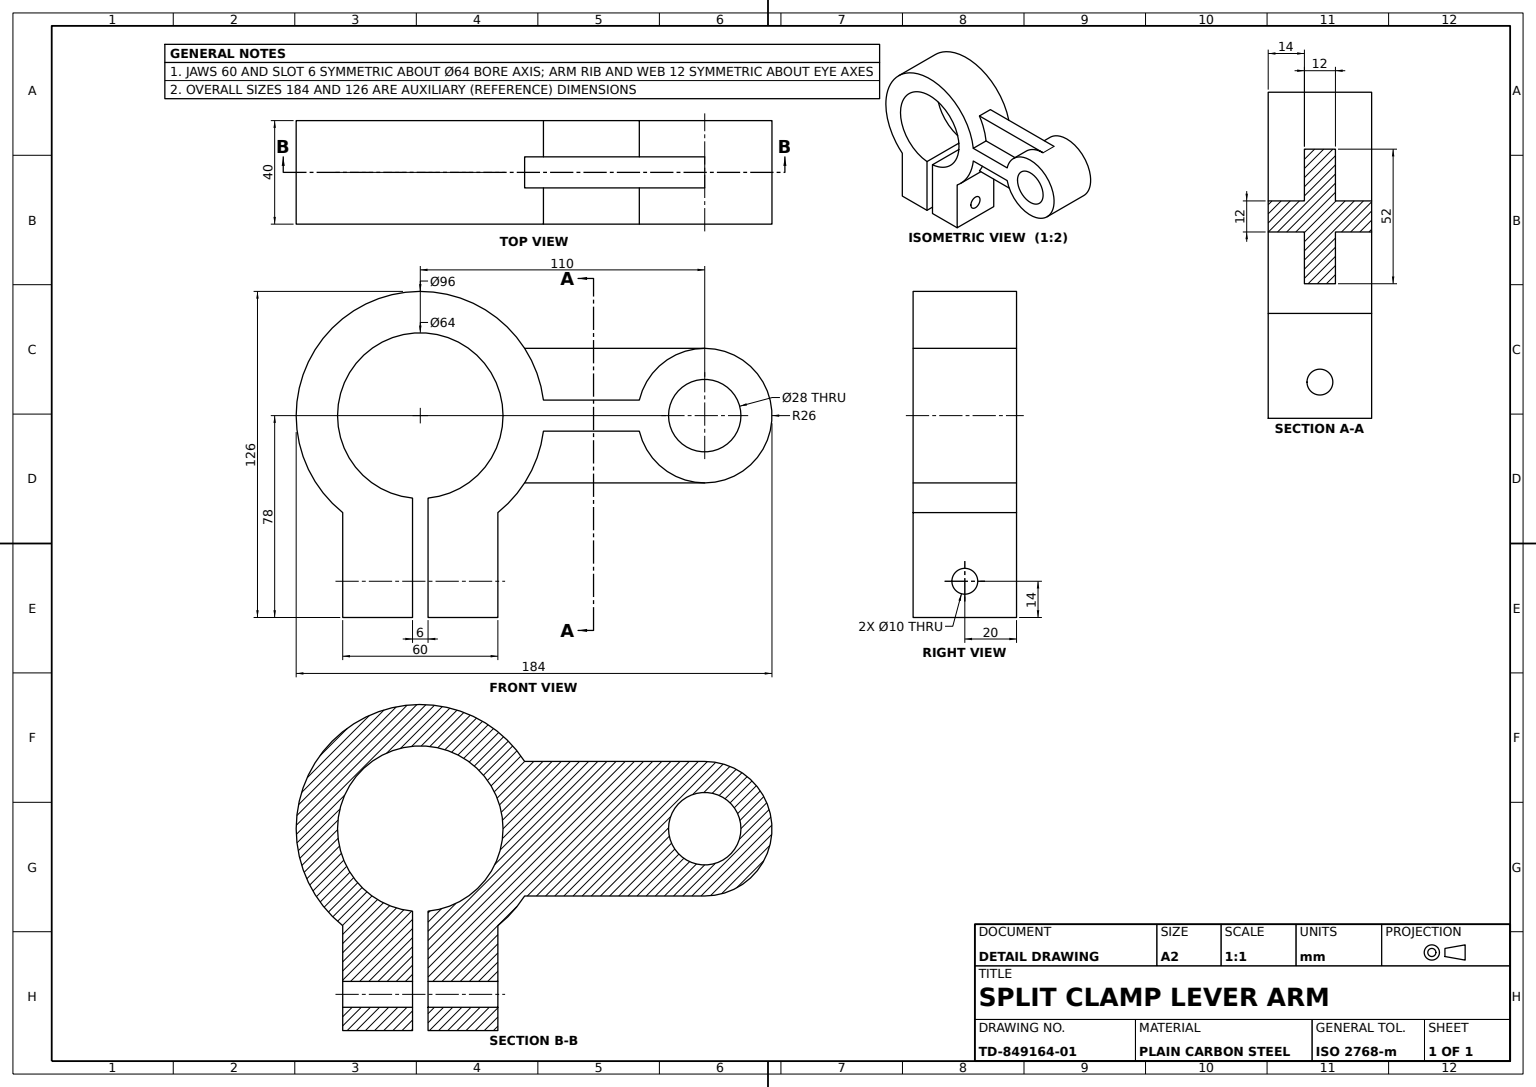
SolidWorks part; units mm, degrees
material "Plain Carbon Steel"
ref_plane "Front Plane" through (0, 0, 0) normal (0, 0, 1) x (1, 0, 0)
ref_plane "Top Plane" through (0, 0, 0) normal (0, 1, 0) x (1, 0, 0)
ref_plane "Right Plane" through (0, 0, 0) normal (1, 0, 0) x (0, 0, -1)
sketch "Clamp Eye Profile" plane through (0, 0, 0) normal (0, 0, 1) x (1, 0, 0)
  line L0 (-30, 40.53) -> (-30, 0)
  line L2 (3, 0) -> (30, 0)
  line L3 (3, 0) -> (3, 46.1409)
  line L5 (-3, 0) -> (-3, 46.1409)
  line L8 (30, 40.53) -> (30, 0)
  line L10 (-30, 0) -> (-3, 0)
  arc A0 (30, 40.53) -> (-30, 40.53) centre (0, 78) ccw
  arc A1 (3, 46.1409) -> (-3, 46.1409) centre (0, 78) ccw
  dimension "D1" = 96
  dimension "D2" = 78
  dimension "D3" = 64
  dimension "D4" = 60
  dimension "D5" = 6
extrude "Clamp Eye Ø96x40" add sketch "Clamp Eye Profile" along normal mid plane 40
sketch "Arm and Small Eye Profile" plane through (0, 0, 0) normal (0, 0, 1) x (1, 0, 0)
  line L1 (47.6235, 72) -> (84.7018, 72)
  line L2 (47.6235, 84) -> (84.7018, 84)
  arc A0 (84.7018, 72) -> (84.7018, 84) centre (110, 78) ccw
  circle A1 centre (110, 78) radius 14
  arc A2 (47.6235, 72) -> (47.6235, 84) centre (0, 78) ccw
  dimension "D2" = 52
  dimension "D3" = 28
  dimension "D1" = 78
  dimension "D4" = 110
  dimension "D5" = 12
  dimension "D6" = 48
extrude "Arm and Small Eye" add sketch "Arm and Small Eye Profile" along normal mid plane 40
sketch "Clamp Screw Hole Sketch" plane through (30, 0, 0) normal (1, 0, 0) x (0, 0, -1)
  line L0 (-20, 0) -> (20, 0) construction
  line L1 (20, 0) -> (20, 40.53) construction
  circle A0 centre (0, 14) radius 5
  dimension "D3" = 10
  dimension "D1" = 14
  dimension "D2" = 20
extrude "Clamp Screw Hole" cut sketch "Clamp Screw Hole Sketch" against normal blind 60
sketch "Arm Rib 1 Sketch" plane through (0, 0, 0) normal (0, 0, 1) x (1, 0, 0)
  line L0 (110, 104) -> (40.3485, 104)
  arc A0 (84.7018, 72) -> (84.7018, 84) centre (110, 78) ccw construction
  arc A1 (47.6235, 84) -> (-30, 40.53) centre (0, 78) ccw construction
  dimension "D1" = 69.6515
rib "Arm Rib 1" sketch "Arm Rib 1 Sketch" sketch "Arm Rib 1 Sketch" thickness 12 extrusion direction parallel to sketch draft on no parameters "D1"=12
sketch "Arm Rib 2 Sketch" plane through (0, 0, 0) normal (0, 0, 1) x (1, 0, 0)
  line L0 (110, 52) -> (40.3485, 52)
  arc A0 (84.7018, 72) -> (84.7018, 84) centre (110, 78) ccw construction
  arc A1 (30, 40.53) -> (47.6235, 72) centre (0, 78) ccw construction
  dimension "D1" = 69.6515
rib "Arm Rib 2" sketch "Arm Rib 2 Sketch" sketch "Arm Rib 2 Sketch" thickness 12 extrusion direction parallel to sketch draft on no parameters "D1"=12
